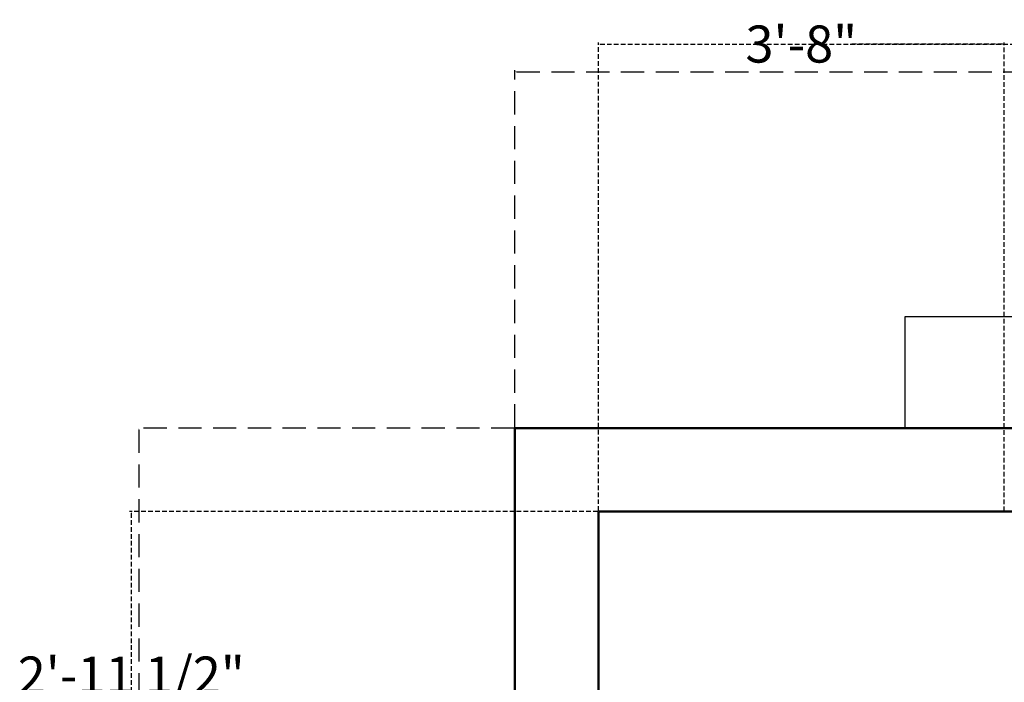
# Model space of a CAD drawing. Units: inches. Extents: x 513 to 1142, y 396 to 927.
# Tile 7 of 31: x 522 to 628, y 852 to 923. Entities that reach past the tile are written whole.
import ezdxf

# ---------------------------------------------------------------- set-up
doc = ezdxf.new("R2010")
doc.units = ezdxf.units.IN
doc.header["$MEASUREMENT"] = 0
doc.linetypes.add('DASHED', pattern=[0.75, 0.5, -0.25])
for name, color, linetype, lineweight in [('A-ANNO-DIMS', 2, 'DASHED', 18), ('A-WALL', 7, 'Continuous', 50), ('windows', 172, 'Continuous', 25)]:
    doc.layers.add(name, color=color, linetype=linetype, lineweight=lineweight)
doc.styles.get("Standard").update_dxf_attribs({"font": 'arial.ttf'})
doc.dimstyles.get("Standard").update_dxf_attribs({"dimtxt": 4, "dimasz": 0.18, "dimexe": 0.18, "dimexo": 0.0625, "dimgap": 0.09, "dimtad": 0, "dimtih": 1, "dimtoh": 1, "dimdec": 0, "dimrnd": 6, "dimzin": 0, "dimdsep": 46, "dimlunit": 3, "dimtxsty": 'Standard', "dimcen": 0.09, "dimadec": 0, "dimazin": 0, "dimtfac": 1, "dimtdec": 0, "dimtofl": 0, "dimtmove": 0, "dimatfit": 3, "dimfxl": 1, "dimtolj": 1, "dimtzin": 0, "dimarcsym": 0})

# ---------------------------------------------------------------- blocks, each defined once
blk = doc.blocks.new('*D103')
at = {"layer": 'A-ANNO-DIMS', "color": 0, "lineweight": -2, "ltscale": 5, "transparency": 16777216}
for p, q in [((575, 879.22), (575, 917.74)), ((575.18, 917.56), (828.93, 917.56)), ((1089.82, 917.56), (836.06, 917.56)), ((1090, 879.22), (1090, 917.74))]:
    blk.add_line(p, q, dxfattribs=at)
at = {"layer": 'A-ANNO-DIMS', "color": 0, "ltscale": 5, "transparency": 16777216}
for points in [[(575.18, 917.59), (575.18, 917.53), (575, 917.56)], [(1089.82, 917.59), (1089.82, 917.53), (1090, 917.56)]]:
    blk.add_solid(points, dxfattribs=at)
at = {"layer": 'Defpoints', "color": 0, "ltscale": 5, "transparency": 16777216}
for p in [(1090, 917.56), (575, 879.16), (1090, 879.16)]:
    blk.add_point(p, dxfattribs=at)
at = {"layer": 'A-ANNO-DIMS', "color": 0, "ltscale": 5, "transparency": 16777216, "insert": (832.5, 917.56), "char_height": 4, "attachment_point": 5}
blk.add_mtext("\\A1;43'", dxfattribs=at)
blk = doc.blocks.new('*D104')
at = {"layer": 'A-ANNO-DIMS', "color": 0, "lineweight": -2, "ltscale": 5, "transparency": 16777216}
for p, q in [((574.93, 879.16), (534.25, 879.16)), ((534.43, 878.98), (534.43, 657.29)), ((534.43, 431.34), (534.43, 653.02)), ((574.93, 431.16), (534.25, 431.16))]:
    blk.add_line(p, q, dxfattribs=at)
at = {"layer": 'A-ANNO-DIMS', "color": 0, "ltscale": 5, "transparency": 16777216}
for points in [[(534.4, 878.98), (534.46, 878.98), (534.43, 879.16)], [(534.4, 431.34), (534.46, 431.34), (534.43, 431.16)]]:
    blk.add_solid(points, dxfattribs=at)
at = {"layer": 'Defpoints', "color": 0, "ltscale": 5, "transparency": 16777216}
for p in [(575, 879.16), (534.43, 431.16), (575, 431.16)]:
    blk.add_point(p, dxfattribs=at)
at = {"layer": 'A-ANNO-DIMS', "color": 0, "ltscale": 5, "transparency": 16777216, "insert": (534.43, 655.16), "char_height": 4, "attachment_point": 5}
blk.add_mtext('\\A1;37\'-6"', dxfattribs=at)
blk = doc.blocks.new('*D135')
at = {"layer": 'A-ANNO-DIMS', "color": 0, "lineweight": -2, "transparency": 16777216}
for p, q in [((584, 870.22), (584, 920.74)), ((584.18, 920.56), (655.22, 920.56)), ((739.82, 920.56), (668.77, 920.56)), ((740, 870.22), (740, 920.74))]:
    blk.add_line(p, q, dxfattribs=at)
at = {"layer": 'A-ANNO-DIMS', "color": 0, "transparency": 16777216}
for points in [[(584.18, 920.59), (584.18, 920.53), (584, 920.56)], [(739.82, 920.59), (739.82, 920.53), (740, 920.56)]]:
    blk.add_solid(points, dxfattribs=at)
at = {"layer": 'Defpoints', "color": 0, "transparency": 16777216}
for p in [(740, 920.56), (584, 870.16), (740, 870.16)]:
    blk.add_point(p, dxfattribs=at)
at = {"layer": 'A-ANNO-DIMS', "color": 0, "transparency": 16777216, "insert": (662, 920.56), "char_height": 4, "attachment_point": 5}
blk.add_mtext('\\A1;13\'-0"', dxfattribs=at)
blk = doc.blocks.new('*D139')
at = {"layer": 'A-ANNO-DIMS', "color": 0, "lineweight": -2, "transparency": 16777216}
for p, q in [((583.93, 870.16), (533.42, 870.16)), ((533.6, 869.98), (533.6, 794.29)), ((533.6, 714.34), (533.6, 790.02)), ((583.93, 714.16), (533.42, 714.16))]:
    blk.add_line(p, q, dxfattribs=at)
at = {"layer": 'A-ANNO-DIMS', "color": 0, "transparency": 16777216}
for points in [[(533.57, 869.98), (533.63, 869.98), (533.6, 870.16)], [(533.57, 714.34), (533.63, 714.34), (533.6, 714.16)]]:
    blk.add_solid(points, dxfattribs=at)
at = {"layer": 'Defpoints', "color": 0, "transparency": 16777216}
for p in [(533.6, 870.16), (584, 870.16), (584, 714.16)]:
    blk.add_point(p, dxfattribs=at)
at = {"layer": 'A-ANNO-DIMS', "color": 0, "transparency": 16777216, "insert": (533.6, 792.16), "char_height": 4, "attachment_point": 5}
blk.add_mtext('\\A1;13\'-0"', dxfattribs=at)
blk = doc.blocks.new('*D152')
at = {"layer": 'A-ANNO-DIMS', "color": 0, "lineweight": -2, "transparency": 16777216}
for p, q in [((584, 870.22), (584, 920.74)), ((584.18, 920.56), (600.49, 920.56)), ((627.61, 920.56), (611.3, 920.56)), ((627.79, 870.19), (627.79, 920.74))]:
    blk.add_line(p, q, dxfattribs=at)
at = {"layer": 'A-ANNO-DIMS', "color": 0, "transparency": 16777216}
for points in [[(584.18, 920.59), (584.18, 920.53), (584, 920.56)], [(627.61, 920.59), (627.61, 920.53), (627.79, 920.56)]]:
    blk.add_solid(points, dxfattribs=at)
at = {"layer": 'Defpoints', "color": 0, "transparency": 16777216}
for p in [(627.79, 920.56), (584, 870.16), (627.79, 870.12)]:
    blk.add_point(p, dxfattribs=at)
at = {"layer": 'A-ANNO-DIMS', "color": 0, "transparency": 16777216, "insert": (605.89, 920.56), "char_height": 4, "attachment_point": 5}
blk.add_mtext('\\A1;3\'-8"', dxfattribs=at)
blk = doc.blocks.new('*D159')
at = {"layer": 'A-ANNO-DIMS', "color": 0, "lineweight": -2, "transparency": 16777216}
for p, q in [((583.93, 870.16), (533.42, 870.16)), ((533.6, 869.98), (533.6, 854.68)), ((533.6, 835.06), (533.6, 850.36)), ((584.07, 834.88), (533.42, 834.88))]:
    blk.add_line(p, q, dxfattribs=at)
at = {"layer": 'A-ANNO-DIMS', "color": 0, "transparency": 16777216}
for points in [[(533.57, 869.98), (533.63, 869.98), (533.6, 870.16)], [(533.57, 835.06), (533.63, 835.06), (533.6, 834.88)]]:
    blk.add_solid(points, dxfattribs=at)
at = {"layer": 'Defpoints', "color": 0, "transparency": 16777216}
for p in [(584, 870.16), (533.6, 834.88), (584.13, 834.88)]:
    blk.add_point(p, dxfattribs=at)
at = {"layer": 'A-ANNO-DIMS', "color": 0, "transparency": 16777216, "insert": (533.6, 852.52), "char_height": 4, "attachment_point": 5}
blk.add_mtext('\\A1;2\'-11 1/2"', dxfattribs=at)
blk = doc.blocks.new('*D170')
at = {"layer": 'A-ANNO-DIMS', "color": 0, "lineweight": -2, "transparency": 16777216}
for p, q in [((835.93, 870.16), (533.42, 870.16)), ((533.6, 869.98), (533.6, 848.29)), ((533.6, 822.34), (533.6, 844.03)), ((835.93, 822.16), (533.42, 822.16))]:
    blk.add_line(p, q, dxfattribs=at)
at = {"layer": 'A-ANNO-DIMS', "color": 0, "transparency": 16777216}
for points in [[(533.57, 869.98), (533.63, 869.98), (533.6, 870.16)], [(533.57, 822.34), (533.63, 822.34), (533.6, 822.16)]]:
    blk.add_solid(points, dxfattribs=at)
at = {"layer": 'Defpoints', "color": 0, "transparency": 16777216}
for p in [(533.6, 870.16), (836, 870.16), (836, 822.16)]:
    blk.add_point(p, dxfattribs=at)
at = {"layer": 'A-ANNO-DIMS', "color": 0, "transparency": 16777216, "insert": (533.6, 846.16), "char_height": 4, "attachment_point": 5}
blk.add_mtext('\\A1;4\'-0"', dxfattribs=at)

msp = doc.modelspace()

# ---------------------------------------------------------------- linework, layer by layer
at = {"layer": 'A-WALL'}
for p, q in [((1090, 879.16), (575, 879.16)), ((575, 879.16), (575, 431.16)), ((584, 870.16), (584, 714.16)), ((740, 870.16), (584, 870.16))]:
    msp.add_line(p, q, dxfattribs=at)
at = {"layer": 'windows'}
for p, q in [((617.06, 891.16), (617.06, 879.16)), ((716.56, 891.16), (617.06, 891.16))]:
    msp.add_line(p, q, dxfattribs=at)

# ---------------------------------------------------------------- dimensions: what is measured, and where the dimension line sits
at = {"layer": 'A-ANNO-DIMS'}
for base, p2, picture, middle in [((740, 920.56), (740, 870.16), '*D135', (662, 920.56)), ((627.79, 920.56), (627.79, 870.12), '*D152', (605.89, 920.56))]:
    dim = msp.add_linear_dim(base=base, p1=(584, 870.16), p2=p2, dimstyle='Standard', override={"dimdec": 1, "dimlfac": 1, "dimrnd": 0, "dimzin": 1, "dimdsep": 46, "dimlunit": 4, "dimfrac": 2}, dxfattribs=at)
    dim.commit()
    dim.dimension.update_dxf_attribs({"geometry": picture, "text_midpoint": middle})
at = {"layer": 'A-ANNO-DIMS', "ltscale": 5}
dim = msp.add_linear_dim(base=(1090, 917.56), p1=(575, 879.16), p2=(1090, 879.16), dimstyle='Standard', override={"dimclrd": 0, "dimclre": 0, "dimclrt": 0}, dxfattribs=at)
dim.commit()
dim.dimension.update_dxf_attribs({"geometry": '*D103', "text_midpoint": (832.5, 917.56)})
dim = msp.add_linear_dim(base=(534.43, 431.16), p1=(575, 879.16), p2=(575, 431.16), angle=90, dimstyle='Standard', override={"dimclrd": 0, "dimclre": 0, "dimclrt": 0}, dxfattribs=at)
dim.commit()
dim.dimension.update_dxf_attribs({"geometry": '*D104', "text_midpoint": (534.43, 655.16)})
at = {"layer": 'A-ANNO-DIMS'}
for base, p1, p2, picture, middle in [((533.6, 834.88), (584, 870.16), (584.13, 834.88), '*D159', (533.6, 852.52)), ((533.6, 870.16), (584, 714.16), (584, 870.16), '*D139', (533.6, 792.16)), ((533.6, 870.16), (836, 822.16), (836, 870.16), '*D170', (533.6, 846.16))]:
    dim = msp.add_linear_dim(base=base, p1=p1, p2=p2, angle=90, dimstyle='Standard', override={"dimdec": 1, "dimlfac": 1, "dimrnd": 0, "dimzin": 1, "dimdsep": 46, "dimlunit": 4, "dimfrac": 2}, dxfattribs=at)
    dim.commit()
    dim.dimension.update_dxf_attribs({"geometry": picture, "text_midpoint": middle})

doc.saveas('drawing.dxf')
